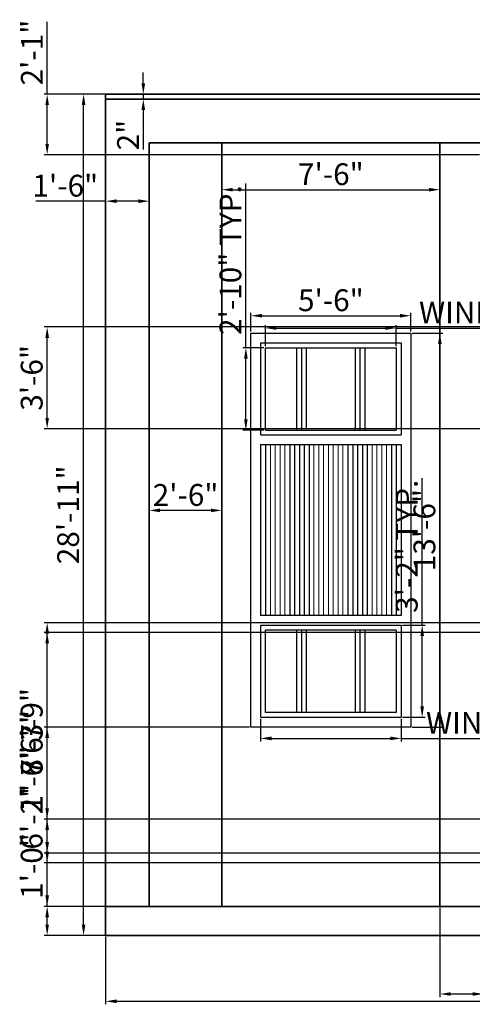
# Model space of a CAD drawing. Units: inches. Extents: x 3297 to 3846, y 520 to 959.
# Tile 1 of 5: x 3297 to 3483, y 524 to 930. Entities that reach past the tile are written whole.
import ezdxf

# ---------------------------------------------------------------- set-up
doc = ezdxf.new("R2010")
doc.units = ezdxf.units.IN
for name, color, linetype, lineweight in [('A-ANNO-DIMS', 2, 'Continuous', 18), ('A-ELEV', 7, 'Continuous', 35), ('A-ELEV-PATT', 8, 'Continuous', 13), ('A-GLAZ', 3, 'Continuous', 25)]:
    doc.layers.add(name, color=color, linetype=linetype, lineweight=lineweight)
doc.styles.get("Standard").update_dxf_attribs({"font": 'arial.ttf'})
doc.dimstyles.new('ISO-25', dxfattribs={"dimtxt": 9, "dimasz": 4.5, "dimexe": 1.25, "dimexo": 0.625, "dimtad": 1, "dimdec": 0, "dimlunit": 3, "dimtxsty": 'Standard', "dimcen": 2.5, "dimadec": 0, "dimazin": 0, "dimtfac": 1, "dimtdec": 0, "dimtmove": 0, "dimatfit": 3, "dimfxl": 1, "dimarcsym": 0})

# ---------------------------------------------------------------- blocks, each defined once
blk = doc.blocks.new('*D5')
at = {"layer": 'A-ANNO-DIMS', "color": 0, "lineweight": -2, "transparency": 16777216}
for p, q in [((3332.06, 878.62), (3332.06, 853.86)), ((3350.06, 878.62), (3350.06, 853.86)), ((3332.06, 855.11), (3303.24, 855.11)), ((3345.56, 855.11), (3336.56, 855.11))]:
    blk.add_line(p, q, dxfattribs=at)
at = {"layer": 'A-ANNO-DIMS', "color": 0, "transparency": 16777216}
for points in [[(3336.56, 855.86), (3336.56, 854.36), (3332.06, 855.11)], [(3345.56, 855.86), (3345.56, 854.36), (3350.06, 855.11)]]:
    blk.add_solid(points, dxfattribs=at)
at = {"layer": 'Defpoints', "color": 0, "transparency": 16777216}
for p in [(3332.06, 879.24), (3350.06, 879.24), (3332.06, 855.11)]:
    blk.add_point(p, dxfattribs=at)
at = {"layer": 'A-ANNO-DIMS', "color": 0, "transparency": 16777216, "insert": (3315.4, 860.33), "char_height": 9, "attachment_point": 5}
blk.add_mtext('1\'-6"', dxfattribs=at)
blk = doc.blocks.new('*D6')
at = {"layer": 'A-ANNO-DIMS', "color": 0, "lineweight": -2, "transparency": 16777216}
for p, q in [((3392.06, 801.31), (3392.06, 809.11)), ((3458.06, 801.31), (3458.06, 809.11)), ((3396.56, 807.86), (3453.56, 807.86))]:
    blk.add_line(p, q, dxfattribs=at)
at = {"layer": 'A-ANNO-DIMS', "color": 0, "transparency": 16777216}
for points in [[(3396.56, 808.61), (3396.56, 807.11), (3392.06, 807.86)], [(3453.56, 808.61), (3453.56, 807.11), (3458.06, 807.86)]]:
    blk.add_solid(points, dxfattribs=at)
at = {"layer": 'Defpoints', "color": 0, "transparency": 16777216}
for p in [(3458.06, 807.86), (3392.06, 800.68), (3458.06, 800.68)]:
    blk.add_point(p, dxfattribs=at)
at = {"layer": 'A-ANNO-DIMS', "color": 0, "transparency": 16777216, "insert": (3425.06, 813.08), "char_height": 9, "attachment_point": 5}
blk.add_mtext('5\'-6"', dxfattribs=at)
blk = doc.blocks.new('*D7')
at = {"layer": 'A-ANNO-DIMS', "color": 0, "lineweight": -2, "transparency": 16777216}
for p, q in [((3332.06, 551.62), (3332.06, 523.84)), ((3737.06, 551.62), (3737.06, 523.84)), ((3336.56, 525.09), (3732.56, 525.09))]:
    blk.add_line(p, q, dxfattribs=at)
at = {"layer": 'A-ANNO-DIMS', "color": 0, "transparency": 16777216}
for points in [[(3336.56, 525.84), (3336.56, 524.34), (3332.06, 525.09)], [(3732.56, 525.84), (3732.56, 524.34), (3737.06, 525.09)]]:
    blk.add_solid(points, dxfattribs=at)
at = {"layer": 'Defpoints', "color": 0, "transparency": 16777216}
for p in [(3332.06, 552.24), (3737.06, 552.24), (3737.06, 525.09)]:
    blk.add_point(p, dxfattribs=at)
at = {"layer": 'A-ANNO-DIMS', "color": 0, "transparency": 16777216, "insert": (3534.56, 530.31), "char_height": 9, "attachment_point": 5}
blk.add_mtext('33\'-9"', dxfattribs=at)
blk = doc.blocks.new('*D8')
at = {"layer": 'A-ANNO-DIMS', "color": 0, "lineweight": -2, "transparency": 16777216}
for p, q in [((3331.44, 899.24), (3321.7, 899.24)), ((3322.95, 556.74), (3322.95, 894.74)), ((3331.44, 552.24), (3321.7, 552.24))]:
    blk.add_line(p, q, dxfattribs=at)
at = {"layer": 'A-ANNO-DIMS', "color": 0, "transparency": 16777216}
for points in [[(3322.2, 894.74), (3323.7, 894.74), (3322.95, 899.24)], [(3322.2, 556.74), (3323.7, 556.74), (3322.95, 552.24)]]:
    blk.add_solid(points, dxfattribs=at)
at = {"layer": 'Defpoints', "color": 0, "transparency": 16777216}
for p in [(3322.95, 899.24), (3332.06, 899.24), (3332.06, 552.24)]:
    blk.add_point(p, dxfattribs=at)
at = {"layer": 'A-ANNO-DIMS', "color": 0, "transparency": 16777216, "insert": (3317.73, 725.74), "char_height": 9, "attachment_point": 5, "rotation": 90}
blk.add_mtext('28\'-11"', dxfattribs=at)
blk = doc.blocks.new('*D9')
at = {"layer": 'A-ANNO-DIMS', "color": 0, "lineweight": -2, "transparency": 16777216}
for p, q in [((3350.06, 765.59), (3350.06, 726.3)), ((3380.06, 765.59), (3380.06, 726.3)), ((3375.56, 727.55), (3354.56, 727.55))]:
    blk.add_line(p, q, dxfattribs=at)
at = {"layer": 'A-ANNO-DIMS', "color": 0, "transparency": 16777216}
for points in [[(3354.56, 728.3), (3354.56, 726.8), (3350.06, 727.55)], [(3375.56, 728.3), (3375.56, 726.8), (3380.06, 727.55)]]:
    blk.add_solid(points, dxfattribs=at)
at = {"layer": 'Defpoints', "color": 0, "transparency": 16777216}
for p in [(3350.06, 766.22), (3380.06, 766.22), (3350.06, 727.55)]:
    blk.add_point(p, dxfattribs=at)
at = {"layer": 'A-ANNO-DIMS', "color": 0, "transparency": 16777216, "insert": (3365.06, 732.77), "char_height": 9, "attachment_point": 5}
blk.add_mtext('2\'-6"', dxfattribs=at)
blk = doc.blocks.new('*D10')
at = {"layer": 'A-ANNO-DIMS', "color": 0, "lineweight": -2, "transparency": 16777216}
for p, q in [((3380.06, 878.62), (3380.06, 858.6)), ((3470.06, 878.62), (3470.06, 858.6)), ((3384.56, 859.85), (3465.56, 859.85))]:
    blk.add_line(p, q, dxfattribs=at)
at = {"layer": 'A-ANNO-DIMS', "color": 0, "transparency": 16777216}
for points in [[(3384.56, 860.6), (3384.56, 859.1), (3380.06, 859.85)], [(3465.56, 860.6), (3465.56, 859.1), (3470.06, 859.85)]]:
    blk.add_solid(points, dxfattribs=at)
at = {"layer": 'Defpoints', "color": 0, "transparency": 16777216}
for p in [(3380.06, 879.24), (3470.06, 879.24), (3470.06, 859.85)]:
    blk.add_point(p, dxfattribs=at)
at = {"layer": 'A-ANNO-DIMS', "color": 0, "transparency": 16777216, "insert": (3425.06, 865.07), "char_height": 9, "attachment_point": 5}
blk.add_mtext('7\'-6"', dxfattribs=at)
blk = doc.blocks.new('*D14')
at = {"layer": 'A-ANNO-DIMS', "color": 0, "lineweight": -2, "transparency": 16777216}
for p, q in [((3458.69, 800.68), (3471.31, 800.68)), ((3470.06, 796.18), (3470.06, 642.71)), ((3458.69, 638.21), (3471.31, 638.21))]:
    blk.add_line(p, q, dxfattribs=at)
at = {"layer": 'A-ANNO-DIMS', "color": 0, "transparency": 16777216}
for points in [[(3469.31, 796.18), (3470.81, 796.18), (3470.06, 800.68)], [(3469.31, 642.71), (3470.81, 642.71), (3470.06, 638.21)]]:
    blk.add_solid(points, dxfattribs=at)
at = {"layer": 'Defpoints', "color": 0, "transparency": 16777216}
for p in [(3458.06, 800.68), (3458.06, 638.21), (3470.06, 638.21)]:
    blk.add_point(p, dxfattribs=at)
at = {"layer": 'A-ANNO-DIMS', "color": 0, "transparency": 16777216, "insert": (3464.84, 719.44), "char_height": 9, "attachment_point": 5, "rotation": 90}
blk.add_mtext('13\'-6"', dxfattribs=at)
blk = doc.blocks.new('*D15')
at = {"layer": 'A-ANNO-DIMS', "color": 0, "lineweight": -2, "transparency": 16777216}
for p, q in [((3347.61, 903.74), (3347.61, 908.24)), ((3332.69, 899.24), (3348.86, 899.24)), ((3347.61, 899.24), (3347.61, 897.24)), ((3332.69, 897.24), (3348.86, 897.24)), ((3347.61, 892.74), (3347.61, 876.49))]:
    blk.add_line(p, q, dxfattribs=at)
at = {"layer": 'A-ANNO-DIMS', "color": 0, "transparency": 16777216}
for points in [[(3346.86, 903.74), (3348.36, 903.74), (3347.61, 899.24)], [(3346.86, 892.74), (3348.36, 892.74), (3347.61, 897.24)]]:
    blk.add_solid(points, dxfattribs=at)
at = {"layer": 'Defpoints', "color": 0, "transparency": 16777216}
for p in [(3332.06, 899.24), (3332.06, 897.24), (3347.61, 897.24)]:
    blk.add_point(p, dxfattribs=at)
at = {"layer": 'A-ANNO-DIMS', "color": 0, "transparency": 16777216, "insert": (3342.47, 882.37), "char_height": 9, "attachment_point": 5, "rotation": 90}
blk.add_mtext('2"', dxfattribs=at)
blk = doc.blocks.new('WIN-FRAME-1200')
for p, q in [((0, 38), (58, 38)), ((0, 0), (0, 38)), ((58, 38), (58, 0)), ((0, 0), (58, 0))]:
    blk.add_line(p, q)
blk = doc.blocks.new('WIN-SASH-1200')
for p, q in [((0, 34), (54, 34)), ((0, 0), (0, 34)), ((54, 34), (54, 0)), ((0, 0), (54, 0))]:
    blk.add_line(p, q)
blk = doc.blocks.new('*D31')
at = {"layer": 'A-ANNO-DIMS', "color": 0, "lineweight": -2, "transparency": 16777216}
for p, q in [((3396.06, 641.58), (3396.06, 632.26)), ((3454.06, 641.58), (3454.06, 632.26)), ((3400.56, 633.51), (3449.56, 633.51)), ((3454.06, 633.51), (3628.19, 633.51))]:
    blk.add_line(p, q, dxfattribs=at)
at = {"layer": 'A-ANNO-DIMS', "color": 0, "transparency": 16777216}
for points in [[(3400.56, 634.26), (3400.56, 632.76), (3396.06, 633.51)], [(3449.56, 634.26), (3449.56, 632.76), (3454.06, 633.51)]]:
    blk.add_solid(points, dxfattribs=at)
at = {"layer": 'Defpoints', "color": 0, "transparency": 16777216}
for p in [(3396.06, 642.21), (3454.06, 642.21), (3454.06, 633.51)]:
    blk.add_point(p, dxfattribs=at)
at = {"layer": 'A-ANNO-DIMS', "color": 0, "transparency": 16777216, "insert": (3543.38, 638.79), "char_height": 9, "attachment_point": 5}
blk.add_mtext('WINDOW FRAME 4\'-10" TYP.', dxfattribs=at)
blk = doc.blocks.new('*D32')
at = {"layer": 'A-ANNO-DIMS', "color": 0, "lineweight": -2, "transparency": 16777216}
for p, q in [((3462.76, 680.21), (3462.76, 740.81)), ((3454.69, 680.21), (3464.01, 680.21)), ((3462.76, 646.71), (3462.76, 675.71)), ((3454.69, 642.21), (3464.01, 642.21))]:
    blk.add_line(p, q, dxfattribs=at)
at = {"layer": 'A-ANNO-DIMS', "color": 0, "transparency": 16777216}
for points in [[(3462.01, 675.71), (3463.51, 675.71), (3462.76, 680.21)], [(3462.01, 646.71), (3463.51, 646.71), (3462.76, 642.21)]]:
    blk.add_solid(points, dxfattribs=at)
at = {"layer": 'Defpoints', "color": 0, "transparency": 16777216}
for p in [(3454.06, 680.21), (3462.76, 680.21), (3454.06, 642.21)]:
    blk.add_point(p, dxfattribs=at)
at = {"layer": 'A-ANNO-DIMS', "color": 0, "transparency": 16777216, "insert": (3457.54, 712.76), "char_height": 9, "attachment_point": 5, "rotation": 90}
blk.add_mtext('3\'-2" TYP.', dxfattribs=at)
blk = doc.blocks.new('*D33')
at = {"layer": 'A-ANNO-DIMS', "color": 0, "lineweight": -2, "transparency": 16777216}
for p, q in [((3398.06, 795.31), (3398.06, 804.03)), ((3402.56, 802.78), (3447.56, 802.78)), ((3452.06, 795.31), (3452.06, 804.03)), ((3452.06, 802.78), (3609.43, 802.78))]:
    blk.add_line(p, q, dxfattribs=at)
at = {"layer": 'A-ANNO-DIMS', "color": 0, "transparency": 16777216}
for points in [[(3402.56, 803.53), (3402.56, 802.03), (3398.06, 802.78)], [(3447.56, 803.53), (3447.56, 802.03), (3452.06, 802.78)]]:
    blk.add_solid(points, dxfattribs=at)
at = {"layer": 'Defpoints', "color": 0, "transparency": 16777216}
for p in [(3452.06, 802.78), (3398.06, 794.68), (3452.06, 794.68)]:
    blk.add_point(p, dxfattribs=at)
at = {"layer": 'A-ANNO-DIMS', "color": 0, "transparency": 16777216, "insert": (3533, 808.06), "char_height": 9, "attachment_point": 5}
blk.add_mtext('WINDOW SASH 4\'-6" TYP.', dxfattribs=at)
blk = doc.blocks.new('*D34')
at = {"layer": 'A-ANNO-DIMS', "color": 0, "lineweight": -2, "transparency": 16777216}
for p, q in [((3389.96, 794.68), (3389.96, 862.44)), ((3397.44, 794.68), (3388.71, 794.68)), ((3389.96, 765.18), (3389.96, 790.18)), ((3397.44, 760.68), (3388.71, 760.68))]:
    blk.add_line(p, q, dxfattribs=at)
at = {"layer": 'A-ANNO-DIMS', "color": 0, "transparency": 16777216}
for points in [[(3389.21, 790.18), (3390.71, 790.18), (3389.96, 794.68)], [(3389.21, 765.18), (3390.71, 765.18), (3389.96, 760.68)]]:
    blk.add_solid(points, dxfattribs=at)
at = {"layer": 'Defpoints', "color": 0, "transparency": 16777216}
for p in [(3389.96, 794.68), (3398.06, 794.68), (3398.06, 760.68)]:
    blk.add_point(p, dxfattribs=at)
at = {"layer": 'A-ANNO-DIMS', "color": 0, "transparency": 16777216, "insert": (3384.74, 830.81), "char_height": 9, "attachment_point": 5, "rotation": 90}
blk.add_mtext('2\'-10" TYP.', dxfattribs=at)
blk = doc.blocks.new('*D55')
at = {"layer": 'A-ANNO-DIMS', "color": 0, "lineweight": -2, "transparency": 16777216}
for p, q in [((3553.14, 681.24), (3306.66, 681.24)), ((3307.91, 604.74), (3307.91, 676.74)), ((3553.14, 600.24), (3306.66, 600.24))]:
    blk.add_line(p, q, dxfattribs=at)
at = {"layer": 'A-ANNO-DIMS', "color": 0, "transparency": 16777216}
for points in [[(3307.16, 676.74), (3308.66, 676.74), (3307.91, 681.24)], [(3307.16, 604.74), (3308.66, 604.74), (3307.91, 600.24)]]:
    blk.add_solid(points, dxfattribs=at)
at = {"layer": 'Defpoints', "color": 0, "transparency": 16777216}
for p in [(3307.91, 681.24), (3553.76, 681.24), (3553.76, 600.24)]:
    blk.add_point(p, dxfattribs=at)
at = {"layer": 'A-ANNO-DIMS', "color": 0, "transparency": 16777216, "insert": (3302.69, 640.74), "char_height": 9, "attachment_point": 5, "rotation": 90}
blk.add_mtext('6\'-9"', dxfattribs=at)
blk = doc.blocks.new('*D56')
at = {"layer": 'A-ANNO-DIMS', "color": 0, "lineweight": -2, "transparency": 16777216}
for p, q in [((3307.91, 600.24), (3307.91, 629.07)), ((3553.14, 600.24), (3306.66, 600.24)), ((3307.91, 586.74), (3307.91, 595.74)), ((3511.44, 582.24), (3306.66, 582.24))]:
    blk.add_line(p, q, dxfattribs=at)
at = {"layer": 'A-ANNO-DIMS', "color": 0, "transparency": 16777216}
for points in [[(3307.16, 595.74), (3308.66, 595.74), (3307.91, 600.24)], [(3307.16, 586.74), (3308.66, 586.74), (3307.91, 582.24)]]:
    blk.add_solid(points, dxfattribs=at)
at = {"layer": 'Defpoints', "color": 0, "transparency": 16777216}
for p in [(3307.91, 600.24), (3553.76, 600.24), (3512.06, 582.24)]:
    blk.add_point(p, dxfattribs=at)
at = {"layer": 'A-ANNO-DIMS', "color": 0, "transparency": 16777216, "insert": (3302.69, 616.9), "char_height": 9, "attachment_point": 5, "rotation": 90}
blk.add_mtext('1\'-6"', dxfattribs=at)
blk = doc.blocks.new('*D57')
at = {"layer": 'A-ANNO-DIMS', "color": 0, "lineweight": -2, "transparency": 16777216}
for p, q in [((3645.44, 681.24), (3306.66, 681.24)), ((3307.91, 586.74), (3307.91, 676.74)), ((3645.44, 582.24), (3306.66, 582.24))]:
    blk.add_line(p, q, dxfattribs=at)
at = {"layer": 'A-ANNO-DIMS', "color": 0, "transparency": 16777216}
for points in [[(3307.16, 676.74), (3308.66, 676.74), (3307.91, 681.24)], [(3307.16, 586.74), (3308.66, 586.74), (3307.91, 582.24)]]:
    blk.add_solid(points, dxfattribs=at)
at = {"layer": 'Defpoints', "color": 0, "transparency": 16777216}
for p in [(3307.91, 681.24), (3646.06, 681.24), (3646.06, 582.24)]:
    blk.add_point(p, dxfattribs=at)
at = {"layer": 'A-ANNO-DIMS', "color": 0, "transparency": 16777216, "insert": (3302.69, 631.74), "char_height": 9, "attachment_point": 5, "rotation": 90}
blk.add_mtext('8\'-3"', dxfattribs=at)
blk = doc.blocks.new('*D59')
at = {"layer": 'A-ANNO-DIMS', "color": 0, "lineweight": -2, "transparency": 16777216}
for p, q in [((3649.439671, 677.241209), (3306.664671, 677.241209)), ((3307.914671, 590.741209), (3307.914671, 672.741209)), ((3649.439671, 586.241209), (3306.664671, 586.241209))]:
    blk.add_line(p, q, dxfattribs=at)
at = {"layer": 'A-ANNO-DIMS', "color": 0, "transparency": 16777216}
for points in [[(3307.164671, 672.741209), (3308.664671, 672.741209), (3307.914671, 677.241209)], [(3307.164671, 590.741209), (3308.664671, 590.741209), (3307.914671, 586.241209)]]:
    blk.add_solid(points, dxfattribs=at)
at = {"layer": 'Defpoints', "color": 0, "transparency": 16777216}
for p in [(3307.914671, 677.241209), (3650.064671, 677.241209), (3650.064671, 586.241209)]:
    blk.add_point(p, dxfattribs=at)
at = {"layer": 'A-ANNO-DIMS', "color": 0, "transparency": 16777216, "insert": (3302.789671, 631.741209), "char_height": 9, "attachment_point": 5, "rotation": 90}
blk.add_mtext('7\'-7"', dxfattribs=at)
blk = doc.blocks.new('*D72')
at = {"layer": 'A-ANNO-DIMS', "color": 0, "lineweight": -2, "transparency": 16777216}
for p, q in [((3555.14, 803.24), (3306.66, 803.24)), ((3307.91, 765.74), (3307.91, 798.74)), ((3555.14, 761.24), (3306.66, 761.24))]:
    blk.add_line(p, q, dxfattribs=at)
at = {"layer": 'A-ANNO-DIMS', "color": 0, "transparency": 16777216}
for points in [[(3307.16, 798.74), (3308.66, 798.74), (3307.91, 803.24)], [(3307.16, 765.74), (3308.66, 765.74), (3307.91, 761.24)]]:
    blk.add_solid(points, dxfattribs=at)
at = {"layer": 'Defpoints', "color": 0, "transparency": 16777216}
for p in [(3307.91, 803.24), (3555.76, 803.24), (3555.76, 761.24)]:
    blk.add_point(p, dxfattribs=at)
at = {"layer": 'A-ANNO-DIMS', "color": 0, "transparency": 16777216, "insert": (3302.69, 782.24), "char_height": 9, "attachment_point": 5, "rotation": 90}
blk.add_mtext('3\'-6"', dxfattribs=at)
blk = doc.blocks.new('*D77')
at = {"layer": 'A-ANNO-DIMS', "color": 0, "lineweight": -2, "transparency": 16777216}
for p, q in [((3470.06, 563.62), (3470.06, 526.84)), ((3488.06, 563.62), (3488.06, 526.84)), ((3474.56, 528.09), (3483.56, 528.09)), ((3488.06, 528.09), (3516.89, 528.09))]:
    blk.add_line(p, q, dxfattribs=at)
at = {"layer": 'A-ANNO-DIMS', "color": 0, "transparency": 16777216}
for points in [[(3474.56, 528.84), (3474.56, 527.34), (3470.06, 528.09)], [(3483.56, 528.84), (3483.56, 527.34), (3488.06, 528.09)]]:
    blk.add_solid(points, dxfattribs=at)
at = {"layer": 'Defpoints', "color": 0, "transparency": 16777216}
for p in [(3470.06, 564.24), (3488.06, 564.24), (3488.06, 528.09)]:
    blk.add_point(p, dxfattribs=at)
at = {"layer": 'A-ANNO-DIMS', "color": 0, "transparency": 16777216, "insert": (3504.73, 533.31), "char_height": 9, "attachment_point": 5}
blk.add_mtext('1\'-6"', dxfattribs=at)
blk = doc.blocks.new('*D78')
at = {"layer": 'A-ANNO-DIMS', "color": 0, "lineweight": -2, "transparency": 16777216}
for p, q in [((3307.91, 899.24), (3307.91, 929.07)), ((3513.44, 899.24), (3306.66, 899.24)), ((3307.91, 878.74), (3307.91, 894.74)), ((3486.44, 874.24), (3306.66, 874.24))]:
    blk.add_line(p, q, dxfattribs=at)
at = {"layer": 'A-ANNO-DIMS', "color": 0, "transparency": 16777216}
for points in [[(3307.16, 894.74), (3308.66, 894.74), (3307.91, 899.24)], [(3307.16, 878.74), (3308.66, 878.74), (3307.91, 874.24)]]:
    blk.add_solid(points, dxfattribs=at)
at = {"layer": 'Defpoints', "color": 0, "transparency": 16777216}
for p in [(3307.91, 899.24), (3514.06, 899.24), (3487.06, 874.24)]:
    blk.add_point(p, dxfattribs=at)
at = {"layer": 'A-ANNO-DIMS', "color": 0, "transparency": 16777216, "insert": (3302.77, 916.41), "char_height": 9, "attachment_point": 5, "rotation": 90}
blk.add_mtext('2\'-1"', dxfattribs=at)
blk = doc.blocks.new('*D79')
at = {"layer": 'A-ANNO-DIMS', "color": 0, "lineweight": -2, "transparency": 16777216}
for p, q in [((3307.91, 564.24), (3307.91, 593.07)), ((3487.44, 564.24), (3306.66, 564.24)), ((3307.91, 556.74), (3307.91, 559.74)), ((3487.44, 552.24), (3306.66, 552.24))]:
    blk.add_line(p, q, dxfattribs=at)
at = {"layer": 'A-ANNO-DIMS', "color": 0, "transparency": 16777216}
for points in [[(3307.16, 559.74), (3308.66, 559.74), (3307.91, 564.24)], [(3307.16, 556.74), (3308.66, 556.74), (3307.91, 552.24)]]:
    blk.add_solid(points, dxfattribs=at)
at = {"layer": 'Defpoints', "color": 0, "transparency": 16777216}
for p in [(3307.91, 564.24), (3488.06, 564.24), (3488.06, 552.24)]:
    blk.add_point(p, dxfattribs=at)
at = {"layer": 'A-ANNO-DIMS', "color": 0, "transparency": 16777216, "insert": (3302.69, 580.9), "char_height": 9, "attachment_point": 5, "rotation": 90}
blk.add_mtext('1\'-0"', dxfattribs=at)
blk = doc.blocks.new('*D80')
at = {"layer": 'A-ANNO-DIMS', "color": 0, "lineweight": -2, "transparency": 16777216}
for p, q in [((3391.44, 638.21), (3306.66, 638.21)), ((3307.91, 568.74), (3307.91, 633.71)), ((3379.44, 564.24), (3306.66, 564.24))]:
    blk.add_line(p, q, dxfattribs=at)
at = {"layer": 'A-ANNO-DIMS', "color": 0, "transparency": 16777216}
for points in [[(3307.16, 633.71), (3308.66, 633.71), (3307.91, 638.21)], [(3307.16, 568.74), (3308.66, 568.74), (3307.91, 564.24)]]:
    blk.add_solid(points, dxfattribs=at)
at = {"layer": 'Defpoints', "color": 0, "transparency": 16777216}
for p in [(3307.91, 638.21), (3392.06, 638.21), (3380.06, 564.24)]:
    blk.add_point(p, dxfattribs=at)
at = {"layer": 'A-ANNO-DIMS', "color": 0, "transparency": 16777216, "insert": (3302.69, 601.22), "char_height": 9, "attachment_point": 5, "rotation": 90}
blk.add_mtext('6\'-2"', dxfattribs=at)

msp = doc.modelspace()

# ---------------------------------------------------------------- linework, layer by layer
at = {"layer": 'A-ELEV'}
for p, q in [((3332.06, 552.24), (3332.06, 899.24)), ((3332.06, 899.24), (3514.06, 899.24)), ((3332.06, 897.24), (3514.06, 897.24)), ((3350.06, 564.24), (3350.06, 879.24)), ((3350.06, 879.24), (3512.06, 879.24)), ((3380.06, 564.24), (3380.06, 879.24)), ((3470.06, 564.24), (3470.06, 879.24)), ((3332.06, 564.24), (3488.06, 564.24)), ((3332.06, 552.24), (3737.06, 552.24))]:
    msp.add_line(p, q, dxfattribs=at)
at = {"layer": 'A-ELEV-PATT'}
for p, q in [((3400.06, 754.68), (3400.06, 684.21)), ((3402.06, 754.68), (3402.06, 684.21)), ((3404.06, 754.68), (3404.06, 684.21)), ((3406.06, 754.68), (3406.06, 684.21)), ((3418.06, 754.68), (3418.06, 684.21)), ((3420.06, 754.68), (3420.06, 684.21)), ((3422.06, 754.68), (3422.06, 684.21)), ((3424.06, 754.68), (3424.06, 684.21)), ((3426.06, 754.68), (3426.06, 684.21)), ((3428.06, 754.68), (3428.06, 684.21)), ((3430.06, 754.68), (3430.06, 684.21)), ((3442.06, 754.68), (3442.06, 684.21)), ((3444.06, 754.68), (3444.06, 684.21)), ((3446.06, 754.68), (3446.06, 684.21)), ((3448.06, 754.68), (3448.06, 684.21))]:
    msp.add_line(p, q, dxfattribs=at)
at = {"layer": 'A-GLAZ'}
for p, q in [((3411.06, 760.68), (3411.06, 794.68)), ((3413.06, 760.68), (3413.06, 794.68)), ((3415.06, 760.68), (3415.06, 794.68)), ((3435.06, 794.68), (3435.06, 760.68)), ((3437.06, 794.68), (3437.06, 760.68)), ((3439.06, 794.68), (3439.06, 760.68)), ((3396.06, 754.68), (3454.06, 754.68)), ((3396.06, 754.68), (3396.06, 684.21)), ((3398.06, 754.68), (3398.06, 684.21)), ((3408.06, 754.68), (3408.06, 684.21)), ((3410.06, 754.68), (3410.06, 684.21)), ((3412.06, 754.68), (3412.06, 684.21)), ((3414.06, 754.68), (3414.06, 684.21)), ((3416.06, 754.68), (3416.06, 684.21)), ((3432.06, 754.68), (3432.06, 684.21)), ((3434.06, 754.68), (3434.06, 684.21)), ((3436.06, 754.68), (3436.06, 684.21)), ((3438.06, 754.68), (3438.06, 684.21)), ((3440.06, 754.68), (3440.06, 684.21)), ((3450.06, 754.68), (3450.06, 684.21)), ((3452.06, 754.68), (3452.06, 684.21)), ((3454.06, 754.68), (3454.06, 684.21)), ((3454.06, 684.21), (3396.06, 684.21)), ((3411.06, 644.21), (3411.06, 678.21)), ((3413.06, 644.21), (3413.06, 678.21)), ((3415.06, 644.21), (3415.06, 678.21)), ((3435.06, 678.21), (3435.06, 644.21)), ((3437.06, 678.21), (3437.06, 644.21)), ((3439.06, 678.21), (3439.06, 644.21))]:
    msp.add_line(p, q, dxfattribs=at)
msp.add_lwpolyline([(3392.06, 800.68), (3458.06, 800.68), (3458.06, 638.21), (3392.06, 638.21)], close=True, dxfattribs=at)

# ---------------------------------------------------------------- block references
for name, p in [('WIN-FRAME-1200', (3396.07, 758.68)), ('WIN-SASH-1200', (3398.07, 760.68)), ('WIN-FRAME-1200', (3396.07, 642.21))]:
    msp.add_blockref(name, p, dxfattribs=at)
at = {"layer": 'A-GLAZ', "rotation": 180}
msp.add_blockref('WIN-SASH-1200', (3452.06, 678.21), dxfattribs=at)

# ---------------------------------------------------------------- dimensions: what is measured, and where the dimension line sits
at = {"layer": 'A-ANNO-DIMS'}
for base, p1, p2, override, picture, middle in [((3307.91, 899.24), (3487.06, 874.24), (3514.06, 899.24), {"dimdec": 1, "dimlfac": 1, "dimrnd": 0, "dimzin": 1, "dimdsep": 46, "dimlunit": 4, "dimfrac": 2}, '*D78', (3302.77, 916.41)), ((3347.61, 897.24), (3332.06, 899.24), (3332.06, 897.24), {"dimclrd": 0, "dimclre": 0, "dimclrt": 0}, '*D15', (3342.47, 882.37)), ((3322.95, 899.24), (3332.06, 552.24), (3332.06, 899.24), {"dimclrd": 0, "dimclre": 0, "dimclrt": 0}, '*D8', (3317.73, 725.74)), ((3307.91, 803.24), (3555.76, 761.24), (3555.76, 803.24), {"dimdec": 1, "dimlfac": 1, "dimrnd": 0, "dimzin": 1, "dimdsep": 46, "dimlunit": 4, "dimfrac": 2}, '*D72', (3302.69, 782.24)), ((3470.06, 638.21), (3458.06, 800.68), (3458.06, 638.21), {"dimclrd": 0, "dimclre": 0, "dimclrt": 0}, '*D14', (3464.84, 719.44)), ((3307.91, 681.24), (3553.76, 600.24), (3553.76, 681.24), {"dimdec": 1, "dimlfac": 1, "dimrnd": 0, "dimzin": 1, "dimdsep": 46, "dimlunit": 4, "dimfrac": 2}, '*D55', (3302.69, 640.74)), ((3307.91, 681.24), (3646.06, 582.24), (3646.06, 681.24), {"dimdec": 1, "dimlfac": 1, "dimrnd": 0, "dimzin": 1, "dimdsep": 46, "dimlunit": 4, "dimfrac": 2}, '*D57', (3302.69, 631.74)), ((3307.91, 677.24), (3650.06, 586.24), (3650.06, 677.24), {"dimdec": 1, "dimlfac": 1, "dimrnd": 0, "dimzin": 1, "dimdsep": 46, "dimlunit": 4, "dimfrac": 2}, '*D59', (3302.79, 631.74)), ((3307.91, 638.21), (3380.06, 564.24), (3392.06, 638.21), {"dimdec": 1, "dimlfac": 1, "dimrnd": 0, "dimzin": 1, "dimdsep": 46, "dimlunit": 4, "dimfrac": 2}, '*D80', (3302.69, 601.22)), ((3307.91, 600.24), (3512.06, 582.24), (3553.76, 600.24), {"dimdec": 1, "dimlfac": 1, "dimrnd": 0, "dimzin": 1, "dimdsep": 46, "dimlunit": 4, "dimfrac": 2}, '*D56', (3302.69, 616.9)), ((3307.91, 564.24), (3488.06, 552.24), (3488.06, 564.24), {"dimdec": 1, "dimlfac": 1, "dimrnd": 0, "dimzin": 1, "dimdsep": 46, "dimlunit": 4, "dimfrac": 2}, '*D79', (3302.69, 580.9))]:
    dim = msp.add_linear_dim(base=base, p1=p1, p2=p2, angle=90, dimstyle='ISO-25', override=override, dxfattribs=at)
    dim.commit()
    dim.dimension.update_dxf_attribs({"geometry": picture, "text_midpoint": middle})
for base, p1, p2, override, picture, middle in [((3332.06, 855.11), (3350.06, 879.24), (3332.06, 879.24), {"dimclrd": 0, "dimclre": 0, "dimclrt": 0}, '*D5', (3315.4, 860.33)), ((3470.06, 859.85), (3380.06, 879.24), (3470.06, 879.24), {"dimclrd": 0, "dimclre": 0, "dimclrt": 0}, '*D10', (3425.06, 865.07)), ((3458.06, 807.86), (3392.06, 800.68), (3458.06, 800.68), {"dimclrd": 0, "dimclre": 0, "dimclrt": 0}, '*D6', (3425.06, 813.08)), ((3350.06, 727.55), (3380.06, 766.22), (3350.06, 766.22), {"dimclrd": 0, "dimclre": 0, "dimclrt": 0}, '*D9', (3365.06, 732.77)), ((3488.06, 528.09), (3470.06, 564.24), (3488.06, 564.24), {"dimdec": 1, "dimlfac": 1, "dimrnd": 0, "dimzin": 1, "dimdsep": 46, "dimlunit": 4, "dimfrac": 2}, '*D77', (3504.73, 533.31)), ((3737.06, 525.09), (3332.06, 552.24), (3737.06, 552.24), {"dimclrd": 0, "dimclre": 0, "dimclrt": 0}, '*D7', (3534.56, 530.31))]:
    dim = msp.add_linear_dim(base=base, p1=p1, p2=p2, dimstyle='ISO-25', override=override, dxfattribs=at)
    dim.commit()
    dim.dimension.update_dxf_attribs({"geometry": picture, "text_midpoint": middle})
for base, p1, p2, picture, middle in [((3389.96, 794.68), (3398.06, 760.68), (3398.06, 794.68), '*D34', (3384.74, 830.81)), ((3462.76, 680.21), (3454.06, 642.21), (3454.06, 680.21), '*D32', (3457.54, 712.76))]:
    dim = msp.add_linear_dim(base=base, p1=p1, p2=p2, angle=90, text='<> TYP.', dimstyle='ISO-25', override={"dimdec": 1, "dimrnd": 0, "dimzin": 1, "dimlunit": 4, "dimfrac": 2}, dxfattribs=at)
    dim.commit()
    dim.dimension.update_dxf_attribs({"geometry": picture, "text_midpoint": middle})
for base, p1, p2, text, picture, middle in [((3452.06, 802.78), (3398.06, 794.68), (3452.06, 794.68), 'WINDOW SASH <> TYP.', '*D33', (3533, 808.06)), ((3454.06, 633.51), (3396.06, 642.21), (3454.06, 642.21), 'WINDOW FRAME <> TYP.', '*D31', (3543.38, 638.79))]:
    dim = msp.add_linear_dim(base=base, p1=p1, p2=p2, text=text, dimstyle='ISO-25', override={"dimdec": 1, "dimrnd": 0, "dimzin": 1, "dimlunit": 4, "dimfrac": 2}, dxfattribs=at)
    dim.commit()
    dim.dimension.update_dxf_attribs({"geometry": picture, "text_midpoint": middle})

doc.saveas('drawing.dxf')
